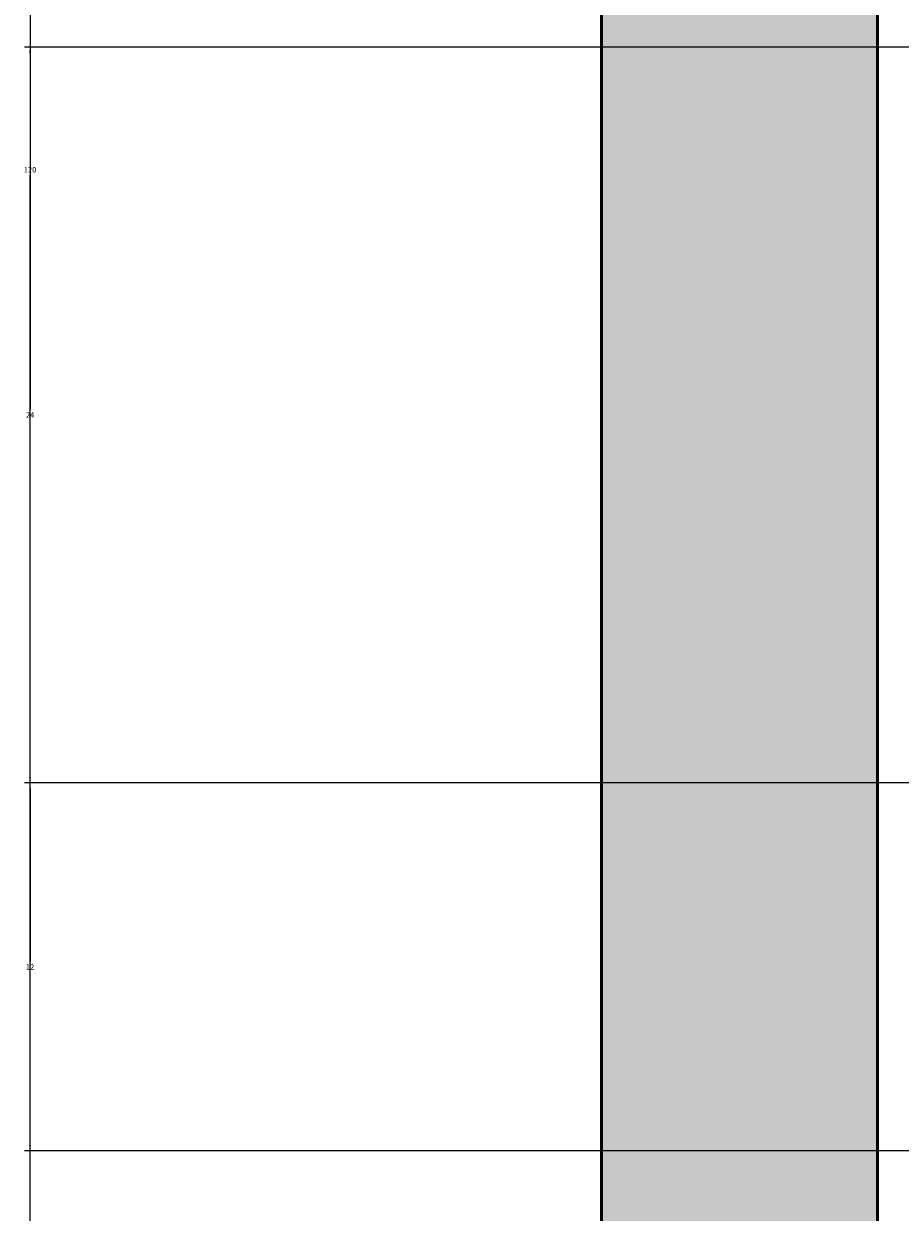
# Model space of a CAD drawing. Units: inches. Extents: x 2231 to 2461, y 2045 to 2455.
# Tile 69 of 95: x 2231 to 2260, y 2333 to 2372. Entities that reach past the tile are written whole.
import ezdxf

# ---------------------------------------------------------------- set-up
doc = ezdxf.new("R2010")
doc.units = ezdxf.units.IN
doc.layers.add('A-ANNO-DIMS', color=2, linetype='Continuous', lineweight=18)
doc.layers.add('A-WALL', color=7, linetype='Continuous', lineweight=50)
doc.layers.add('A-WALL-PATT', color=18, linetype='Continuous', lineweight=13, true_color=0x000000)
doc.styles.get("Standard").update_dxf_attribs({"font": 'arial.ttf'})
doc.dimstyles.get("Standard").update_dxf_attribs({"dimtxt": 0.18, "dimasz": 0.18, "dimexe": 0.18, "dimexo": 0.0625, "dimgap": 0.09, "dimtad": 0, "dimtih": 1, "dimtoh": 1, "dimdec": 4, "dimzin": 0, "dimdsep": 46, "dimtxsty": 'Standard', "dimcen": 0.09, "dimadec": 0, "dimazin": 0, "dimtfac": 1, "dimtdec": 4, "dimtofl": 0, "dimtmove": 0, "dimatfit": 3, "dimfxl": 1, "dimtolj": 1, "dimtzin": 0, "dimarcsym": 0})

# ---------------------------------------------------------------- blocks, each defined once
blk = doc.blocks.new('*D37')
at = {"layer": 'A-ANNO-DIMS', "color": 0, "lineweight": -2, "transparency": 16777216}
for p, q in [((2258.731, 2426.833), (2230.981, 2426.833)), ((2231.161, 2426.653), (2231.161, 2367.015)), ((2231.161, 2307.013), (2231.161, 2366.651)), ((2258.731, 2306.833), (2230.981, 2306.833))]:
    blk.add_line(p, q, dxfattribs=at)
at = {"layer": 'A-ANNO-DIMS', "color": 0, "transparency": 16777216}
for points in [[(2231.131, 2426.653), (2231.191, 2426.653), (2231.161, 2426.833)], [(2231.131, 2307.013), (2231.191, 2307.013), (2231.161, 2306.833)]]:
    blk.add_solid(points, dxfattribs=at)
at = {"layer": 'Defpoints', "color": 0, "transparency": 16777216}
for p in [(2231.161, 2426.833), (2258.794, 2426.833), (2258.794, 2306.833)]:
    blk.add_point(p, dxfattribs=at)
at = {"layer": 'A-ANNO-DIMS', "color": 0, "transparency": 16777216, "insert": (2231.161, 2366.833), "char_height": 0.18, "attachment_point": 5}
blk.add_mtext('\\A1;120', dxfattribs=at)
blk = doc.blocks.new('*D47')
at = {"layer": 'A-ANNO-DIMS', "color": 0, "lineweight": -2, "transparency": 16777216}
for p, q in [((2258.794, 2182.895), (2258.794, 2454.645)), ((2258.974, 2454.465), (2276.575, 2454.465)), ((2294.614, 2454.465), (2277.012, 2454.465)), ((2294.794, 2182.895), (2294.794, 2454.645))]:
    blk.add_line(p, q, dxfattribs=at)
at = {"layer": 'A-ANNO-DIMS', "color": 0, "transparency": 16777216}
for points in [[(2258.974, 2454.495), (2258.974, 2454.435), (2258.794, 2454.465)], [(2294.614, 2454.495), (2294.614, 2454.435), (2294.794, 2454.465)]]:
    blk.add_solid(points, dxfattribs=at)
at = {"layer": 'Defpoints', "color": 0, "transparency": 16777216}
for p in [(2294.794, 2454.465), (2258.794, 2182.833), (2294.794, 2182.833)]:
    blk.add_point(p, dxfattribs=at)
at = {"layer": 'A-ANNO-DIMS', "color": 0, "transparency": 16777216, "insert": (2276.794, 2454.465), "char_height": 0.18, "attachment_point": 5}
blk.add_mtext('\\A1;36', dxfattribs=at)
blk = doc.blocks.new('*D53')
at = {"layer": 'A-ANNO-DIMS', "color": 0, "lineweight": -2, "transparency": 16777216}
for p, q in [((2372.731, 2346.833), (2230.981, 2346.833)), ((2231.161, 2346.653), (2231.161, 2341.013)), ((2231.161, 2335.013), (2231.161, 2340.652)), ((2372.731, 2334.833), (2230.981, 2334.833))]:
    blk.add_line(p, q, dxfattribs=at)
at = {"layer": 'A-ANNO-DIMS', "color": 0, "transparency": 16777216}
for points in [[(2231.131, 2346.653), (2231.191, 2346.653), (2231.161, 2346.833)], [(2231.131, 2335.013), (2231.191, 2335.013), (2231.161, 2334.833)]]:
    blk.add_solid(points, dxfattribs=at)
at = {"layer": 'Defpoints', "color": 0, "transparency": 16777216}
for p in [(2231.161, 2346.833), (2372.794, 2346.833), (2372.794, 2334.833)]:
    blk.add_point(p, dxfattribs=at)
at = {"layer": 'A-ANNO-DIMS', "color": 0, "transparency": 16777216, "insert": (2231.161, 2340.833), "char_height": 0.18, "attachment_point": 5}
blk.add_mtext('\\A1;12', dxfattribs=at)
blk = doc.blocks.new('*D54')
at = {"layer": 'A-ANNO-DIMS', "color": 0, "lineweight": -2, "transparency": 16777216}
for p, q in [((2372.731, 2370.833), (2230.981, 2370.833)), ((2231.161, 2370.653), (2231.161, 2359.013)), ((2231.161, 2347.013), (2231.161, 2358.652)), ((2372.731, 2346.833), (2230.981, 2346.833))]:
    blk.add_line(p, q, dxfattribs=at)
at = {"layer": 'A-ANNO-DIMS', "color": 0, "transparency": 16777216}
for points in [[(2231.131, 2370.653), (2231.191, 2370.653), (2231.161, 2370.833)], [(2231.131, 2347.013), (2231.191, 2347.013), (2231.161, 2346.833)]]:
    blk.add_solid(points, dxfattribs=at)
at = {"layer": 'Defpoints', "color": 0, "transparency": 16777216}
for p in [(2231.161, 2370.833), (2372.794, 2370.833), (2372.794, 2346.833)]:
    blk.add_point(p, dxfattribs=at)
at = {"layer": 'A-ANNO-DIMS', "color": 0, "transparency": 16777216, "insert": (2231.161, 2358.833), "char_height": 0.18, "attachment_point": 5}
blk.add_mtext('\\A1;24', dxfattribs=at)

msp = doc.modelspace()

# ---------------------------------------------------------------- hatches: boundary and pattern name
at = {"layer": 'A-WALL-PATT'}
h = msp.add_hatch(color=256, dxfattribs=at)
h.dxf.hatch_style = 1
h.paths.add_polyline_path([(2441.7935, 2269.1535), (2432.7935, 2269.1535), (2432.7935, 2186.8328), (2396.7935, 2186.8328), (2396.7935, 2286.8328), (2394.7935, 2286.8328), (2394.7935, 2186.8328), (2334.7935, 2186.8328), (2334.7935, 2182.8328), (2432.7935, 2182.8328), (2432.7935, 2072.8328), (2416.6639, 2072.8328), (2416.6639, 2063.8328), (2441.7935, 2063.8328)])
h.paths.add_polyline_path([(2368.6639, 2072.8328), (2367.04, 2072.8328), (2330.7942, 2072.8328), (2330.7397, 2063.8328), (2368.6639, 2063.8328)])
h.paths.add_polyline_path([(2300.7392, 2068.3328), (2300.7392, 2072.8328), (2298.7935, 2072.8328), (2294.7935, 2072.8328), (2258.7935, 2072.8328), (2258.7935, 2120.8328), (2294.7935, 2120.8328), (2298.7935, 2120.8328), (2298.7935, 2128.8328), (2294.7935, 2128.8328), (2294.7935, 2124.8328), (2258.7935, 2124.8328), (2258.7935, 2182.8328), (2294.7935, 2182.8328), (2294.7935, 2174.8328), (2298.7935, 2174.8328), (2298.7935, 2182.8328), (2304.7935, 2182.8328), (2304.7935, 2186.8328), (2258.7935, 2186.8328), (2258.7935, 2221.999), (2249.7935, 2221.999), (2249.7935, 2063.8328), (2300.7392, 2063.8328)])
h.paths.add_polyline_path([(2391.9338, 2435.8328), (2333.82, 2435.8328), (2333.82, 2426.8328), (2368.7935, 2426.8328), (2368.7935, 2374.9508), (2368.7935, 2370.8328), (2372.3935, 2370.8328), (2372.7935, 2370.8328), (2372.7935, 2426.8328), (2391.9338, 2426.8328)])
h.paths.add_polyline_path([(2441.7935, 2435.8328), (2415.9338, 2435.8328), (2415.9338, 2426.8328), (2432.7935, 2426.8328), (2432.7935, 2334.8328), (2372.7935, 2334.8328), (2372.7935, 2346.8328), (2368.7935, 2346.8328), (2368.7935, 2306.8328), (2360.7935, 2306.8328), (2360.7935, 2302.8328), (2368.7935, 2302.8328), (2372.7935, 2302.8328), (2372.7935, 2330.8328), (2432.7935, 2330.8328), (2432.7935, 2317.1535), (2441.7935, 2317.1535)])
h.paths.add_polyline_path([(2285.82, 2435.8328), (2249.7935, 2435.8328), (2249.7935, 2269.999), (2258.7935, 2269.999), (2258.7935, 2302.8328), (2318.8168, 2302.8328), (2330.7935, 2302.8328), (2330.7935, 2306.8328), (2258.7935, 2306.8328), (2258.7935, 2426.8328), (2285.82, 2426.8328)])

# ---------------------------------------------------------------- linework, layer by layer
at = {"layer": 'A-WALL'}
msp.add_line((2258.7935, 2306.8328), (2258.7935, 2426.8328), dxfattribs=at)
msp.add_lwpolyline([(2300.7392, 2063.8328), (2249.7935, 2063.8328), (2249.7935, 2435.8328), (2441.7935, 2435.8328), (2441.7935, 2063.8328), (2330.7397, 2063.8328)], dxfattribs=at)

# ---------------------------------------------------------------- dimensions: what is measured, and where the dimension line sits
at = {"layer": 'A-ANNO-DIMS'}
dim = msp.add_linear_dim(base=(2294.7935, 2454.4653), p1=(2258.7935, 2182.8328), p2=(2294.7935, 2182.8328), dimstyle='Standard', override={"dimdec": 0, "dimlfac": 1, "dimrnd": 0, "dimzin": 0, "dimdsep": 46, "dimlunit": 2}, dxfattribs=at)
dim.commit()
dim.dimension.update_dxf_attribs({"geometry": '*D47', "text_midpoint": (2276.7935, 2454.4653)})
for base, p1, p2, picture, middle in [((2231.161, 2426.8328), (2258.7935, 2306.8328), (2258.7935, 2426.8328), '*D37', (2231.161, 2366.8328)), ((2231.161, 2370.8328), (2372.7935, 2346.8328), (2372.7935, 2370.8328), '*D54', (2231.161, 2358.8328)), ((2231.161, 2346.8328), (2372.7935, 2334.8328), (2372.7935, 2346.8328), '*D53', (2231.161, 2340.8328))]:
    dim = msp.add_linear_dim(base=base, p1=p1, p2=p2, angle=90, dimstyle='Standard', override={"dimdec": 0, "dimlfac": 1, "dimrnd": 0, "dimzin": 0, "dimdsep": 46, "dimlunit": 2}, dxfattribs=at)
    dim.commit()
    dim.dimension.update_dxf_attribs({"geometry": picture, "text_midpoint": middle})

doc.saveas('drawing.dxf')
